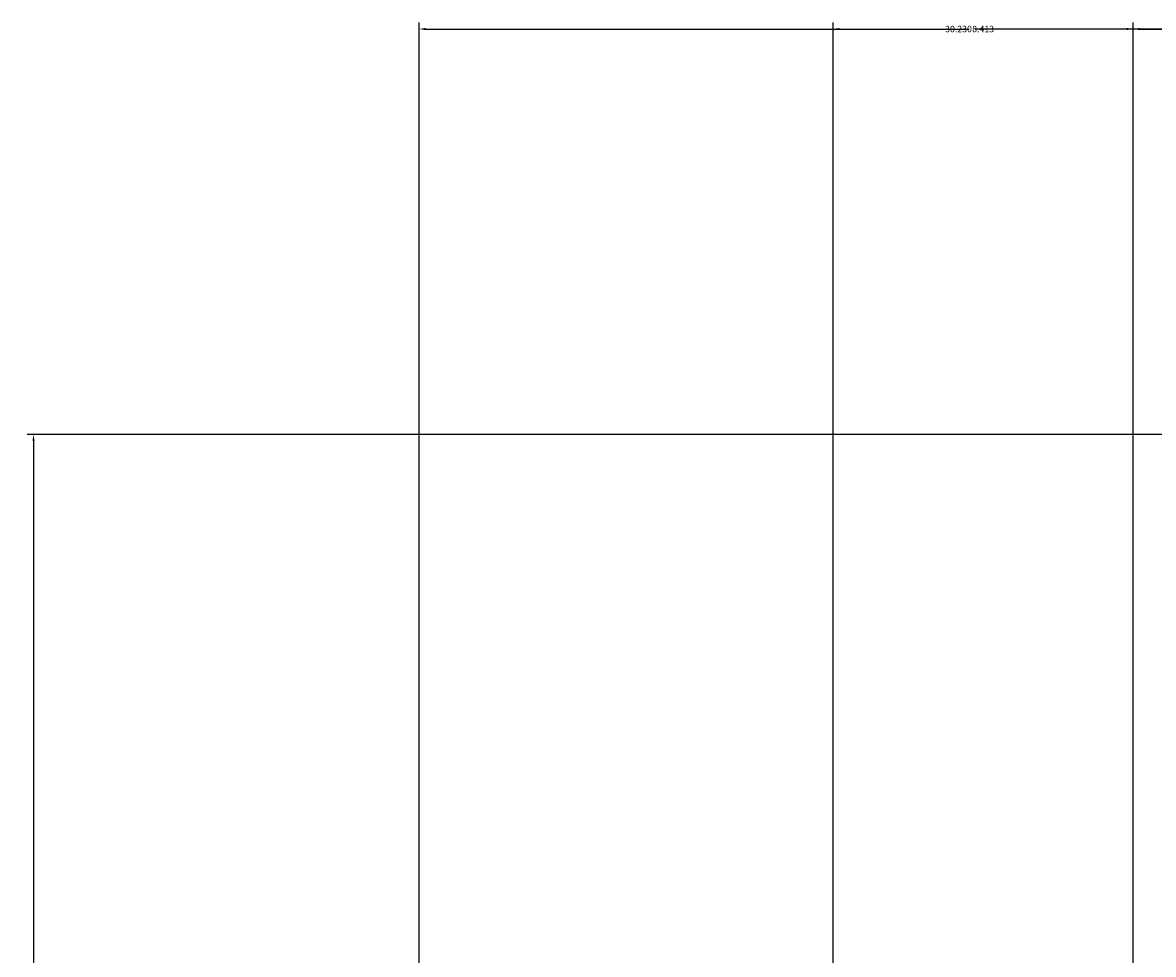
# Model space of a CAD drawing. Units: inches. Extents: x -117 to 121, y -77 to 40.
# Tile 11 of 45: x -117 to -85, y 12 to 39. Entities that reach past the tile are written whole.
import ezdxf

# ---------------------------------------------------------------- set-up
doc = ezdxf.new("R2010")
doc.units = ezdxf.units.IN
doc.header["$MEASUREMENT"] = 0
doc.layers.add('A-ANNO-DIMS', color=2, linetype='Continuous', lineweight=18)
doc.styles.get("Standard").update_dxf_attribs({"font": 'arial.ttf'})
doc.dimstyles.get("Standard").update_dxf_attribs({"dimtxt": 0.18, "dimasz": 0.18, "dimexe": 0.18, "dimexo": 0.0625, "dimgap": 0.09, "dimtad": 0, "dimtih": 1, "dimtoh": 1, "dimdec": 4, "dimzin": 0, "dimdsep": 46, "dimtxsty": 'Standard', "dimcen": 0.09, "dimadec": 0, "dimazin": 0, "dimtfac": 1, "dimtdec": 4, "dimtofl": 0, "dimtmove": 0, "dimatfit": 3, "dimfxl": 1, "dimtolj": 1, "dimtzin": 0, "dimarcsym": 0})

# ---------------------------------------------------------------- blocks, each defined once
blk = doc.blocks.new('*D13')
at = {"layer": 'A-ANNO-DIMS', "color": 0, "lineweight": -2, "transparency": 16777216}
for p, q in [((-2.663, 27.063), (-117.024, 27.063)), ((-116.844, 26.883), (-116.844, -16.974)), ((-116.844, -61.196), (-116.844, -17.338)), ((-106.096, -61.376), (-117.024, -61.376))]:
    blk.add_line(p, q, dxfattribs=at)
at = {"layer": 'A-ANNO-DIMS', "color": 0, "transparency": 16777216}
for points in [[(-116.874, 26.883), (-116.814, 26.883), (-116.844, 27.063)], [(-116.874, -61.196), (-116.814, -61.196), (-116.844, -61.376)]]:
    blk.add_solid(points, dxfattribs=at)
at = {"layer": 'Defpoints', "color": 0, "transparency": 16777216}
for p in [(-2.6, 27.063), (-116.844, -61.376), (-106.034, -61.376)]:
    blk.add_point(p, dxfattribs=at)
at = {"layer": 'A-ANNO-DIMS', "color": 0, "transparency": 16777216, "insert": (-116.844, -17.156), "char_height": 0.18, "attachment_point": 5}
blk.add_mtext('\\A1;88.44', dxfattribs=at)
blk = doc.blocks.new('*D21')
at = {"layer": 'A-ANNO-DIMS', "color": 0, "lineweight": -2, "transparency": 16777216}
for p, q in [((-106.034, -61.313), (-106.034, 38.61)), ((-105.854, 38.43), (-91.382, 38.43)), ((-75.984, 38.43), (-90.455, 38.43)), ((-75.804, 8.087), (-75.804, 38.61))]:
    blk.add_line(p, q, dxfattribs=at)
at = {"layer": 'A-ANNO-DIMS', "color": 0, "transparency": 16777216}
for points in [[(-105.854, 38.46), (-105.854, 38.4), (-106.034, 38.43)], [(-75.984, 38.46), (-75.984, 38.4), (-75.804, 38.43)]]:
    blk.add_solid(points, dxfattribs=at)
at = {"layer": 'Defpoints', "color": 0, "transparency": 16777216}
for p in [(-75.804, 38.43), (-75.804, 8.025), (-106.034, -61.376)]:
    blk.add_point(p, dxfattribs=at)
at = {"layer": 'A-ANNO-DIMS', "color": 0, "transparency": 16777216, "insert": (-90.919, 38.43), "char_height": 0.18, "attachment_point": 5}
blk.add_mtext('\\A1;30.230', dxfattribs=at)
blk = doc.blocks.new('*D39')
at = {"layer": 'A-ANNO-DIMS', "color": 0, "lineweight": -2, "transparency": 16777216}
for p, q in [((-94.436, -12.071), (-94.436, 38.61)), ((-94.256, 38.43), (-90.623, 38.43)), ((-86.203, 38.43), (-89.835, 38.43)), ((-86.023, -13.677), (-86.023, 38.61))]:
    blk.add_line(p, q, dxfattribs=at)
at = {"layer": 'A-ANNO-DIMS', "color": 0, "transparency": 16777216}
for points in [[(-94.256, 38.46), (-94.256, 38.4), (-94.436, 38.43)], [(-86.203, 38.46), (-86.203, 38.4), (-86.023, 38.43)]]:
    blk.add_solid(points, dxfattribs=at)
at = {"layer": 'Defpoints', "color": 0, "transparency": 16777216}
for p in [(-86.023, 38.43), (-94.436, -12.133), (-86.023, -13.74)]:
    blk.add_point(p, dxfattribs=at)
at = {"layer": 'A-ANNO-DIMS', "color": 0, "transparency": 16777216, "insert": (-90.229, 38.43), "char_height": 0.18, "attachment_point": 5}
blk.add_mtext('\\A1;8.413', dxfattribs=at)
blk = doc.blocks.new('*D40')
at = {"layer": 'A-ANNO-DIMS', "color": 0, "lineweight": -2, "transparency": 16777216}
for p, q in [((-86.023, -13.677), (-86.023, 38.61)), ((-85.843, 38.43), (-75.056, 38.43)), ((-63.339, 38.43), (-74.126, 38.43)), ((-63.159, -13.677), (-63.159, 38.61))]:
    blk.add_line(p, q, dxfattribs=at)
at = {"layer": 'A-ANNO-DIMS', "color": 0, "transparency": 16777216}
for points in [[(-85.843, 38.46), (-85.843, 38.4), (-86.023, 38.43)], [(-63.339, 38.46), (-63.339, 38.4), (-63.159, 38.43)]]:
    blk.add_solid(points, dxfattribs=at)
at = {"layer": 'Defpoints', "color": 0, "transparency": 16777216}
for p in [(-63.159, 38.43), (-86.023, -13.74), (-63.159, -13.74)]:
    blk.add_point(p, dxfattribs=at)
at = {"layer": 'A-ANNO-DIMS', "color": 0, "transparency": 16777216, "insert": (-74.591, 38.43), "char_height": 0.18, "attachment_point": 5}
blk.add_mtext('\\A1;22.864', dxfattribs=at)

msp = doc.modelspace()

# ---------------------------------------------------------------- dimensions: what is measured, and where the dimension line sits
at = {"layer": 'A-ANNO-DIMS'}
for base, p1, p2, picture, middle in [((-75.8037, 38.4297), (-106.0338, -61.3756), (-75.8037, 8.0246), '*D21', (-90.9187, 38.4297)), ((-86.0225, 38.4297), (-94.4355, -12.1334), (-86.0225, -13.74), '*D39', (-90.229, 38.4297)), ((-63.1589, 38.4297), (-86.0225, -13.74), (-63.1589, -13.74), '*D40', (-74.5907, 38.4297))]:
    dim = msp.add_linear_dim(base=base, p1=p1, p2=p2, dimstyle='Standard', override={"dimdec": 3, "dimlfac": 1, "dimrnd": 0, "dimzin": 0, "dimdsep": 46, "dimlunit": 2}, dxfattribs=at)
    dim.commit()
    dim.dimension.update_dxf_attribs({"geometry": picture, "text_midpoint": middle})
dim = msp.add_linear_dim(base=(-116.8438, -61.3756), p1=(-2.6001, 27.0634), p2=(-106.0338, -61.3756), angle=90, dimstyle='Standard', override={"dimdec": 2, "dimlfac": 1, "dimrnd": 0, "dimzin": 0, "dimdsep": 46, "dimlunit": 2}, dxfattribs=at)
dim.commit()
dim.dimension.update_dxf_attribs({"geometry": '*D13', "text_midpoint": (-116.8438, -17.1561)})

doc.saveas('drawing.dxf')
